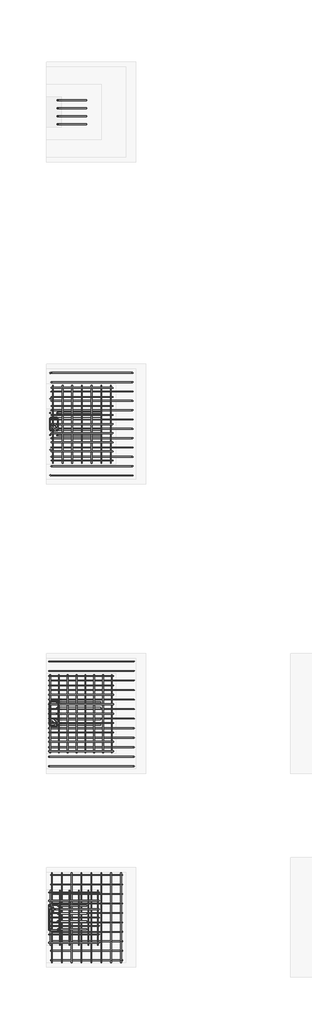
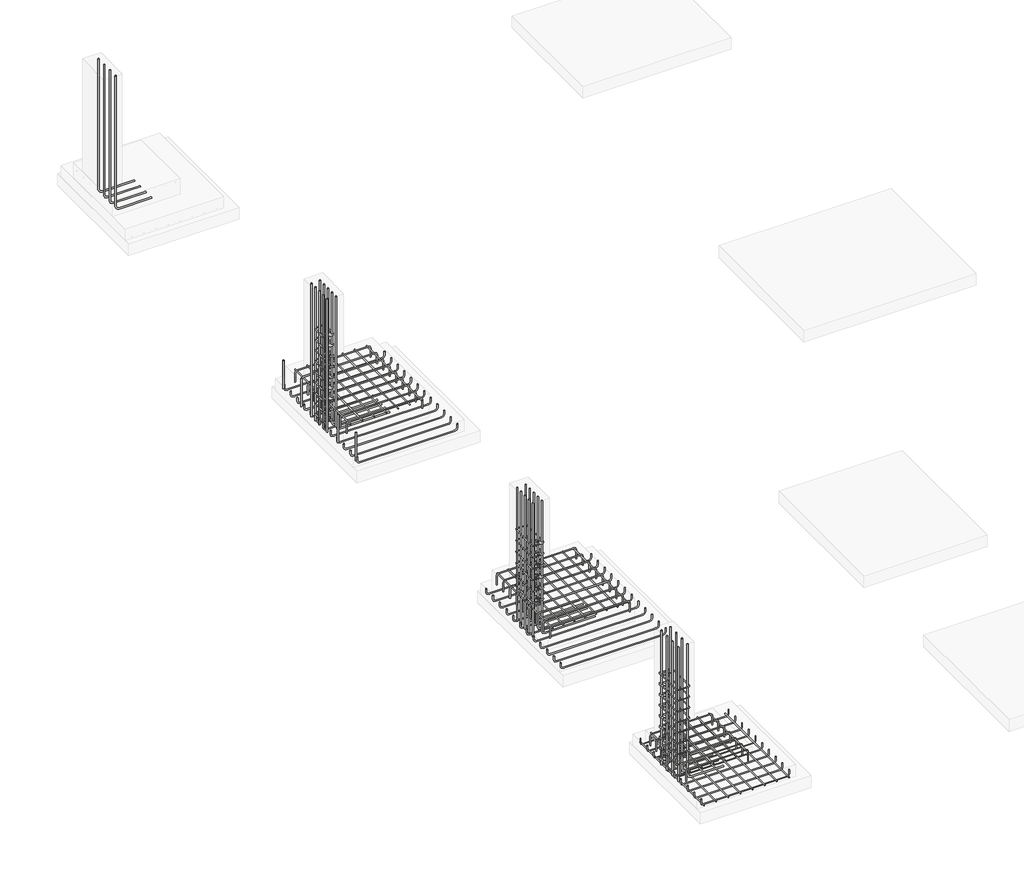
# One storey, part 2 of 6: 21 reinforcing bars.
"""IFC4 building model written with IfcOpenShell, lengths in millimetres."""

from ifc_helpers import new_model, si_unit, point, frame, origin, place, context, project, spatial, polyline, circle_curve, trimmed, segment, composite_curve, source, transform, mapped, element, save
from ifc_brep_helpers import swept_disk

model = new_model("IFC4")

# Units and contexts
model_context = context("Model", 3, world=origin())
ifc_project = project(units=[si_unit("LENGTHUNIT", "METRE", prefix="MILLI")], contexts=[model_context])

# Site, building, storey
site = spatial("IfcSite", under=ifc_project)
building = spatial("IfcBuilding", under=site)
storey = spatial("IfcBuildingStorey", under=building, Elevation=-1828.8)

# Reinforcing bars
placement = place(None, origin())
reinforcing_bar_shape = source(origin(), model_context, "Body", "SolidModel", [
    swept_disk(composite_curve([segment(polyline([(5663595.3113073, -3589696.1284482, -1571.6), (5663595.3113073, -3589696.1284482, -1457.6)]), True, "CONTINUOUS"), segment(trimmed(circle_curve(frame((5663565.3113073, -3589696.1284482, -1457.6), z_axis=(0.0, -1.0, 0.0), x_axis=(30.0, 0.0, 0.0)), 30.0), [point((5663595.3113073, -3589696.1284482, -1457.6))], [point((5663565.3113073, -3589696.1284482, -1427.6))], True, "CARTESIAN"), True, "CONTINUOUS"), segment(polyline([(5663565.3113073, -3589696.1284482, -1427.6), (5662690.0789718, -3589696.1284482, -1427.6)]), True, "CONTINUOUS"), segment(trimmed(circle_curve(frame((5662690.0789718, -3589696.1284482, -1457.6), z_axis=(0.0, -1.0, 0.0), x_axis=(0.0, 0.0, 30.0)), 30.0), [point((5662690.0789718, -3589696.1284482, -1427.6))], [point((5662660.0789718, -3589696.1284482, -1457.6))], True, "CARTESIAN"), True, "CONTINUOUS"), segment(polyline([(5662660.0789718, -3589696.1284482, -1457.6), (5662660.0789718, -3589696.1284482, -1571.6)]), True, "CONTINUOUS")], self_intersect=False), 6.0),
])
element("IfcReinforcingBar", 1, at=placement, inside=storey, context=model_context, shape_type="MappedRepresentation", body=[
    mapped(reinforcing_bar_shape, transform((0.0, 0.0, 0.0), x_axis=(1.0, 0.0, 0.0), y_axis=(0.0, 1.0, 0.0), z_axis=(0.0, 0.0, 1.0))),
    mapped(reinforcing_bar_shape, transform((0.0, -138.4, 0.0), x_axis=(1.0, 0.0, 0.0), y_axis=(0.0, 1.0, 0.0), z_axis=(0.0, 0.0, 1.0))),
    mapped(reinforcing_bar_shape, transform((0.0, -276.8, 0.0), x_axis=(1.0, 0.0, 0.0), y_axis=(0.0, 1.0, 0.0), z_axis=(0.0, 0.0, 1.0))),
    mapped(reinforcing_bar_shape, transform((0.0, -415.2, 0.0), x_axis=(1.0, 0.0, 0.0), y_axis=(0.0, 1.0, 0.0), z_axis=(0.0, 0.0, 1.0))),
    mapped(reinforcing_bar_shape, transform((0.0, -553.6, 0.0), x_axis=(1.0, 0.0, 0.0), y_axis=(0.0, 1.0, 0.0), z_axis=(0.0, 0.0, 1.0))),
    mapped(reinforcing_bar_shape, transform((0.0, -692.0, 0.0), x_axis=(1.0, 0.0, 0.0), y_axis=(0.0, 1.0, 0.0), z_axis=(0.0, 0.0, 1.0))),
    mapped(reinforcing_bar_shape, transform((0.0, -830.4, 0.0), x_axis=(1.0, 0.0, 0.0), y_axis=(0.0, 1.0, 0.0), z_axis=(0.0, 0.0, 1.0))),
    mapped(reinforcing_bar_shape, transform((0.0, -968.8, 0.0), x_axis=(1.0, 0.0, 0.0), y_axis=(0.0, 1.0, 0.0), z_axis=(0.0, 0.0, 1.0))),
    mapped(reinforcing_bar_shape, transform((0.0, -1107.2, 0.0), x_axis=(1.0, 0.0, 0.0), y_axis=(0.0, 1.0, 0.0), z_axis=(0.0, 0.0, 1.0))),
])
reinforcing_bar_2_shape = source(origin(), model_context, "Body", "SolidModel", [
    swept_disk(composite_curve([segment(polyline([(5663568.7965546, -3589656.6584405, -1439.5588801), (5663568.7965546, -3590844.2228659, -1439.5588801)]), True, "CONTINUOUS")], self_intersect=False), 6.0),
])
element("IfcReinforcingBar", 2, at=placement, inside=storey, context=model_context, shape_type="MappedRepresentation", body=[
    mapped(reinforcing_bar_2_shape, transform((0.0, 0.0, 0.0), x_axis=(1.0, 0.0, 0.0), y_axis=(0.0, 1.0, 0.0), z_axis=(0.0, 0.0, 1.0))),
    mapped(reinforcing_bar_2_shape, transform((-147.5988176, 0.0, 0.0), x_axis=(1.0, 0.0, 0.0), y_axis=(0.0, 1.0, 0.0), z_axis=(0.0, 0.0, 1.0))),
    mapped(reinforcing_bar_2_shape, transform((-295.1976351, 0.0, 0.0), x_axis=(1.0, 0.0, 0.0), y_axis=(0.0, 1.0, 0.0), z_axis=(0.0, 0.0, 1.0))),
    mapped(reinforcing_bar_2_shape, transform((-442.7964527, 0.0, 0.0), x_axis=(1.0, 0.0, 0.0), y_axis=(0.0, 1.0, 0.0), z_axis=(0.0, 0.0, 1.0))),
    mapped(reinforcing_bar_2_shape, transform((-590.3952702, 0.0, 0.0), x_axis=(1.0, 0.0, 0.0), y_axis=(0.0, 1.0, 0.0), z_axis=(0.0, 0.0, 1.0))),
    mapped(reinforcing_bar_2_shape, transform((-737.9940878, 0.0, 0.0), x_axis=(1.0, 0.0, 0.0), y_axis=(0.0, 1.0, 0.0), z_axis=(0.0, 0.0, 1.0))),
    mapped(reinforcing_bar_2_shape, transform((-885.5929054, 0.0, 0.0), x_axis=(1.0, 0.0, 0.0), y_axis=(0.0, 1.0, 0.0), z_axis=(0.0, 0.0, 1.0))),
])
reinforcing_bar_3_shape = source(origin(), model_context, "Body", "SolidModel", [
    swept_disk(composite_curve([segment(polyline([(5662620.5113073, -3595238.8523052, -1551.6), (5662620.5113073, -3595238.8523052, -1437.6)]), True, "CONTINUOUS"), segment(trimmed(circle_curve(frame((5662650.5113073, -3595238.8523052, -1437.6), z_axis=(0.0, 1.0, 0.0), x_axis=(-30.0, 0.0, 0.0)), 30.0), [point((5662620.5113073, -3595238.8523052, -1437.6))], [point((5662650.5113073, -3595238.8523052, -1407.6))], True, "CARTESIAN"), True, "CONTINUOUS"), segment(polyline([(5662650.5113073, -3595238.8523052, -1407.6), (5663575.9557483, -3595238.8523052, -1407.6)]), True, "CONTINUOUS"), segment(trimmed(circle_curve(frame((5663575.9557483, -3595238.8523052, -1437.6), z_axis=(0.0, 1.0, 0.0), x_axis=(0.0, 0.0, 30.0)), 30.0), [point((5663575.9557483, -3595238.8523052, -1407.6))], [point((5663605.9557483, -3595238.8523052, -1437.6))], True, "CARTESIAN"), True, "CONTINUOUS"), segment(polyline([(5663605.9557483, -3595238.8523052, -1437.6), (5663605.9557483, -3595238.8523052, -1551.6)]), True, "CONTINUOUS")], self_intersect=False), 6.0),
])
element("IfcReinforcingBar", 3, at=placement, inside=storey, context=model_context, shape_type="MappedRepresentation", body=[
    mapped(reinforcing_bar_3_shape, transform((0.0, 0.0, 0.0), x_axis=(1.0, 0.0, 0.0), y_axis=(0.0, 1.0, 0.0), z_axis=(0.0, 0.0, 1.0))),
    mapped(reinforcing_bar_3_shape, transform((0.0, 143.4, 0.0), x_axis=(1.0, 0.0, 0.0), y_axis=(0.0, 1.0, 0.0), z_axis=(0.0, 0.0, 1.0))),
    mapped(reinforcing_bar_3_shape, transform((0.0, 286.8, 0.0), x_axis=(1.0, 0.0, 0.0), y_axis=(0.0, 1.0, 0.0), z_axis=(0.0, 0.0, 1.0))),
    mapped(reinforcing_bar_3_shape, transform((0.0, 430.2, 0.0), x_axis=(1.0, 0.0, 0.0), y_axis=(0.0, 1.0, 0.0), z_axis=(0.0, 0.0, 1.0))),
    mapped(reinforcing_bar_3_shape, transform((0.0, 573.6, 0.0), x_axis=(1.0, 0.0, 0.0), y_axis=(0.0, 1.0, 0.0), z_axis=(0.0, 0.0, 1.0))),
    mapped(reinforcing_bar_3_shape, transform((0.0, 717.0, 0.0), x_axis=(1.0, 0.0, 0.0), y_axis=(0.0, 1.0, 0.0), z_axis=(0.0, 0.0, 1.0))),
    mapped(reinforcing_bar_3_shape, transform((0.0, 860.4, 0.0), x_axis=(1.0, 0.0, 0.0), y_axis=(0.0, 1.0, 0.0), z_axis=(0.0, 0.0, 1.0))),
    mapped(reinforcing_bar_3_shape, transform((0.0, 1003.8, 0.0), x_axis=(1.0, 0.0, 0.0), y_axis=(0.0, 1.0, 0.0), z_axis=(0.0, 0.0, 1.0))),
    mapped(reinforcing_bar_3_shape, transform((0.0, 1147.2, 0.0), x_axis=(1.0, 0.0, 0.0), y_axis=(0.0, 1.0, 0.0), z_axis=(0.0, 0.0, 1.0))),
])
reinforcing_bar_4_shape = source(origin(), model_context, "Body", "SolidModel", [
    swept_disk(composite_curve([segment(polyline([(5662641.1545158, -3595258.3223129, -1419.7151301), (5662641.1545158, -3594070.7578875, -1419.7151301)]), True, "CONTINUOUS")], self_intersect=False), 6.0),
])
element("IfcReinforcingBar", 4, at=placement, inside=storey, context=model_context, shape_type="MappedRepresentation", body=[
    mapped(reinforcing_bar_4_shape, transform((0.0, 0.0, 0.0), x_axis=(1.0, 0.0, 0.0), y_axis=(0.0, 1.0, 0.0), z_axis=(0.0, 0.0, 1.0))),
    mapped(reinforcing_bar_4_shape, transform((134.3834574, 0.0, 0.0), x_axis=(1.0, 0.0, 0.0), y_axis=(0.0, 1.0, 0.0), z_axis=(0.0, 0.0, 1.0))),
    mapped(reinforcing_bar_4_shape, transform((268.7669147, 0.0, 0.0), x_axis=(1.0, 0.0, 0.0), y_axis=(0.0, 1.0, 0.0), z_axis=(0.0, 0.0, 1.0))),
    mapped(reinforcing_bar_4_shape, transform((403.1503721, 0.0, 0.0), x_axis=(1.0, 0.0, 0.0), y_axis=(0.0, 1.0, 0.0), z_axis=(0.0, 0.0, 1.0))),
    mapped(reinforcing_bar_4_shape, transform((537.5338294, 0.0, 0.0), x_axis=(1.0, 0.0, 0.0), y_axis=(0.0, 1.0, 0.0), z_axis=(0.0, 0.0, 1.0))),
    mapped(reinforcing_bar_4_shape, transform((671.9172868, 0.0, 0.0), x_axis=(1.0, 0.0, 0.0), y_axis=(0.0, 1.0, 0.0), z_axis=(0.0, 0.0, 1.0))),
    mapped(reinforcing_bar_4_shape, transform((806.3007441, 0.0, 0.0), x_axis=(1.0, 0.0, 0.0), y_axis=(0.0, 1.0, 0.0), z_axis=(0.0, 0.0, 1.0))),
    mapped(reinforcing_bar_4_shape, transform((940.6842015, 0.0, 0.0), x_axis=(1.0, 0.0, 0.0), y_axis=(0.0, 1.0, 0.0), z_axis=(0.0, 0.0, 1.0))),
])
reinforcing_bar_5_shape = source(origin(), model_context, "Body", "SolidModel", [
    swept_disk(composite_curve([segment(polyline([(5662620.5113073, -3593868.6554739, -1738.0317047), (5662620.5113073, -3593868.6554739, -1787.0317047)]), True, "CONTINUOUS"), segment(trimmed(circle_curve(frame((5662650.5113073, -3593868.6554739, -1787.0317047), z_axis=(0.0, -1.0, 0.0), x_axis=(-30.0, 0.0, 0.0)), 30.0), [point((5662620.5113073, -3593868.6554739, -1787.0317047))], [point((5662650.5113073, -3593868.6554739, -1817.0317047))], True, "CARTESIAN"), True, "CONTINUOUS"), segment(polyline([(5662650.5113073, -3593868.6554739, -1817.0317047), (5663890.1113073, -3593868.6554739, -1817.0317047)]), True, "CONTINUOUS"), segment(trimmed(circle_curve(frame((5663890.1113073, -3593868.6554739, -1787.0317047), z_axis=(0.0, -1.0, 0.0), x_axis=(0.0, 0.0, -30.0)), 30.0), [point((5663890.1113073, -3593868.6554739, -1817.0317047))], [point((5663920.1113073, -3593868.6554739, -1787.0317047))], True, "CARTESIAN"), True, "CONTINUOUS"), segment(polyline([(5663920.1113073, -3593868.6554739, -1787.0317047), (5663920.1113073, -3593868.6554739, -1738.0317047)]), True, "CONTINUOUS")], self_intersect=False), 6.0),
])
element("IfcReinforcingBar", 5, at=placement, inside=storey, context=model_context, shape_type="MappedRepresentation", body=[
    mapped(reinforcing_bar_5_shape, transform((0.0, 0.0, 0.0), x_axis=(1.0, 0.0, 0.0), y_axis=(0.0, 1.0, 0.0), z_axis=(0.0, 0.0, 1.0))),
    mapped(reinforcing_bar_5_shape, transform((0.0, -145.3451665, 0.0), x_axis=(1.0, 0.0, 0.0), y_axis=(0.0, 1.0, 0.0), z_axis=(0.0, 0.0, 1.0))),
    mapped(reinforcing_bar_5_shape, transform((0.0, -290.690333, 0.0), x_axis=(1.0, 0.0, 0.0), y_axis=(0.0, 1.0, 0.0), z_axis=(0.0, 0.0, 1.0))),
    mapped(reinforcing_bar_5_shape, transform((0.0, -436.0354994, 0.0), x_axis=(1.0, 0.0, 0.0), y_axis=(0.0, 1.0, 0.0), z_axis=(0.0, 0.0, 1.0))),
    mapped(reinforcing_bar_5_shape, transform((0.0, -581.3806659, 0.0), x_axis=(1.0, 0.0, 0.0), y_axis=(0.0, 1.0, 0.0), z_axis=(0.0, 0.0, 1.0))),
    mapped(reinforcing_bar_5_shape, transform((0.0, -726.7258324, 0.0), x_axis=(1.0, 0.0, 0.0), y_axis=(0.0, 1.0, 0.0), z_axis=(0.0, 0.0, 1.0))),
    mapped(reinforcing_bar_5_shape, transform((0.0, -872.0709989, 0.0), x_axis=(1.0, 0.0, 0.0), y_axis=(0.0, 1.0, 0.0), z_axis=(0.0, 0.0, 1.0))),
    mapped(reinforcing_bar_5_shape, transform((0.0, -1017.4161654, 0.0), x_axis=(1.0, 0.0, 0.0), y_axis=(0.0, 1.0, 0.0), z_axis=(0.0, 0.0, 1.0))),
    mapped(reinforcing_bar_5_shape, transform((0.0, -1162.7613318, 0.0), x_axis=(1.0, 0.0, 0.0), y_axis=(0.0, 1.0, 0.0), z_axis=(0.0, 0.0, 1.0))),
    mapped(reinforcing_bar_5_shape, transform((0.0, -1308.1064983, 0.0), x_axis=(1.0, 0.0, 0.0), y_axis=(0.0, 1.0, 0.0), z_axis=(0.0, 0.0, 1.0))),
    mapped(reinforcing_bar_5_shape, transform((0.0, -1453.4516648, 0.0), x_axis=(1.0, 0.0, 0.0), y_axis=(0.0, 1.0, 0.0), z_axis=(0.0, 0.0, 1.0))),
    mapped(reinforcing_bar_5_shape, transform((0.0, -1598.7968313, 0.0), x_axis=(1.0, 0.0, 0.0), y_axis=(0.0, 1.0, 0.0), z_axis=(0.0, 0.0, 1.0))),
])
reinforcing_bar_6_shape = source(origin(), model_context, "Body", "SolidModel", [
    swept_disk(composite_curve([segment(polyline([(5662651.6237213, -3597125.2875145, -1738.4709043), (5662651.6237213, -3597125.2875145, -1793.4709043)]), True, "CONTINUOUS"), segment(trimmed(circle_curve(frame((5662676.6237213, -3597125.2875145, -1793.4709043), z_axis=(0.0, -1.0, 0.0), x_axis=(-25.0, 0.0, 0.0)), 25.0), [point((5662651.6237213, -3597125.2875145, -1793.4709043))], [point((5662676.6237213, -3597125.2875145, -1818.4709043))], True, "CARTESIAN"), True, "CONTINUOUS"), segment(polyline([(5662676.6237213, -3597125.2875145, -1818.4709043), (5663718.1378894, -3597125.2875145, -1818.4709043)]), True, "CONTINUOUS"), segment(trimmed(circle_curve(frame((5663718.1378894, -3597125.2875145, -1793.4709043), z_axis=(0.0, -1.0, 0.0), x_axis=(0.0, 0.0, -25.0)), 25.0), [point((5663718.1378894, -3597125.2875145, -1818.4709043))], [point((5663743.1378894, -3597125.2875145, -1793.4709043))], True, "CARTESIAN"), True, "CONTINUOUS"), segment(polyline([(5663743.1378894, -3597125.2875145, -1793.4709043), (5663743.1378894, -3597125.2875145, -1738.4709043)]), True, "CONTINUOUS")], self_intersect=False), 5.0),
])
element("IfcReinforcingBar", 6, at=placement, inside=storey, context=model_context, shape_type="MappedRepresentation", body=[
    mapped(reinforcing_bar_6_shape, transform((0.0, 0.0, 0.0), x_axis=(1.0, 0.0, 0.0), y_axis=(0.0, 1.0, 0.0), z_axis=(0.0, 0.0, 1.0))),
    mapped(reinforcing_bar_6_shape, transform((0.0, -144.6222222, 0.0), x_axis=(1.0, 0.0, 0.0), y_axis=(0.0, 1.0, 0.0), z_axis=(0.0, 0.0, 1.0))),
    mapped(reinforcing_bar_6_shape, transform((0.0, -289.2444444, 0.0), x_axis=(1.0, 0.0, 0.0), y_axis=(0.0, 1.0, 0.0), z_axis=(0.0, 0.0, 1.0))),
    mapped(reinforcing_bar_6_shape, transform((0.0, -433.8666667, 0.0), x_axis=(1.0, 0.0, 0.0), y_axis=(0.0, 1.0, 0.0), z_axis=(0.0, 0.0, 1.0))),
    mapped(reinforcing_bar_6_shape, transform((0.0, -578.4888889, 0.0), x_axis=(1.0, 0.0, 0.0), y_axis=(0.0, 1.0, 0.0), z_axis=(0.0, 0.0, 1.0))),
    mapped(reinforcing_bar_6_shape, transform((0.0, -723.1111111, 0.0), x_axis=(1.0, 0.0, 0.0), y_axis=(0.0, 1.0, 0.0), z_axis=(0.0, 0.0, 1.0))),
    mapped(reinforcing_bar_6_shape, transform((0.0, -867.7333333, 0.0), x_axis=(1.0, 0.0, 0.0), y_axis=(0.0, 1.0, 0.0), z_axis=(0.0, 0.0, 1.0))),
    mapped(reinforcing_bar_6_shape, transform((0.0, -1012.3555556, 0.0), x_axis=(1.0, 0.0, 0.0), y_axis=(0.0, 1.0, 0.0), z_axis=(0.0, 0.0, 1.0))),
    mapped(reinforcing_bar_6_shape, transform((0.0, -1156.9777778, 0.0), x_axis=(1.0, 0.0, 0.0), y_axis=(0.0, 1.0, 0.0), z_axis=(0.0, 0.0, 1.0))),
    mapped(reinforcing_bar_6_shape, transform((0.0, -1301.6, 0.0), x_axis=(1.0, 0.0, 0.0), y_axis=(0.0, 1.0, 0.0), z_axis=(0.0, 0.0, 1.0))),
])
reinforcing_bar_7_shape = source(origin(), model_context, "Body", "SolidModel", [
    swept_disk(composite_curve([segment(polyline([(5662668.193273, -3597090.2875145, -1807.7638193), (5662668.193273, -3598461.8875145, -1807.7638193)]), True, "CONTINUOUS")], self_intersect=False), 5.0),
])
element("IfcReinforcingBar", 7, at=placement, inside=storey, context=model_context, shape_type="MappedRepresentation", body=[
    mapped(reinforcing_bar_7_shape, transform((0.0, 0.0, 0.0), x_axis=(1.0, 0.0, 0.0), y_axis=(0.0, 1.0, 0.0), z_axis=(0.0, 0.0, 1.0))),
    mapped(reinforcing_bar_7_shape, transform((150.6667583, 0.0, 0.0), x_axis=(1.0, 0.0, 0.0), y_axis=(0.0, 1.0, 0.0), z_axis=(0.0, 0.0, 1.0))),
    mapped(reinforcing_bar_7_shape, transform((301.3335165, 0.0, 0.0), x_axis=(1.0, 0.0, 0.0), y_axis=(0.0, 1.0, 0.0), z_axis=(0.0, 0.0, 1.0))),
    mapped(reinforcing_bar_7_shape, transform((452.0002748, 0.0, 0.0), x_axis=(1.0, 0.0, 0.0), y_axis=(0.0, 1.0, 0.0), z_axis=(0.0, 0.0, 1.0))),
    mapped(reinforcing_bar_7_shape, transform((602.6670331, 0.0, 0.0), x_axis=(1.0, 0.0, 0.0), y_axis=(0.0, 1.0, 0.0), z_axis=(0.0, 0.0, 1.0))),
    mapped(reinforcing_bar_7_shape, transform((753.3337913, 0.0, 0.0), x_axis=(1.0, 0.0, 0.0), y_axis=(0.0, 1.0, 0.0), z_axis=(0.0, 0.0, 1.0))),
    mapped(reinforcing_bar_7_shape, transform((904.0005496, 0.0, 0.0), x_axis=(1.0, 0.0, 0.0), y_axis=(0.0, 1.0, 0.0), z_axis=(0.0, 0.0, 1.0))),
    mapped(reinforcing_bar_7_shape, transform((1054.6673079, 0.0, 0.0), x_axis=(1.0, 0.0, 0.0), y_axis=(0.0, 1.0, 0.0), z_axis=(0.0, 0.0, 1.0))),
])
reinforcing_bar_8_shape = source(origin(), model_context, "Body", "SolidModel", [
    swept_disk(composite_curve([segment(polyline([(5662657.3977763, -3589467.5284482, -1743.8), (5662657.3977763, -3589467.5284482, -1792.8)]), True, "CONTINUOUS"), segment(trimmed(circle_curve(frame((5662687.3977763, -3589467.5284482, -1792.8), z_axis=(0.0, -1.0, 0.0), x_axis=(-30.0, 0.0, 0.0)), 30.0), [point((5662657.3977763, -3589467.5284482, -1792.8))], [point((5662687.3977763, -3589467.5284482, -1822.8))], True, "CARTESIAN"), True, "CONTINUOUS"), segment(polyline([(5662687.3977763, -3589467.5284482, -1822.8), (5663870.1113073, -3589467.5284482, -1822.8)]), True, "CONTINUOUS"), segment(trimmed(circle_curve(frame((5663870.1113073, -3589467.5284482, -1792.8), z_axis=(0.0, -1.0, 0.0), x_axis=(0.0, 0.0, -30.0)), 30.0), [point((5663870.1113073, -3589467.5284482, -1822.8))], [point((5663900.1113073, -3589467.5284482, -1792.8))], True, "CARTESIAN"), True, "CONTINUOUS"), segment(polyline([(5663900.1113073, -3589467.5284482, -1792.8), (5663900.1113073, -3589467.5284482, -1743.8)]), True, "CONTINUOUS")], self_intersect=False), 6.0),
])
element("IfcReinforcingBar", 8, at=placement, inside=storey, context=model_context, shape_type="MappedRepresentation", body=[
    mapped(reinforcing_bar_8_shape, transform((0.0, 0.0, 0.0), x_axis=(1.0, 0.0, 0.0), y_axis=(0.0, 1.0, 0.0), z_axis=(0.0, 0.0, 1.0))),
    mapped(reinforcing_bar_8_shape, transform((0.0, -142.2181818, 0.0), x_axis=(1.0, 0.0, 0.0), y_axis=(0.0, 1.0, 0.0), z_axis=(0.0, 0.0, 1.0))),
    mapped(reinforcing_bar_8_shape, transform((0.0, -284.4363636, 0.0), x_axis=(1.0, 0.0, 0.0), y_axis=(0.0, 1.0, 0.0), z_axis=(0.0, 0.0, 1.0))),
    mapped(reinforcing_bar_8_shape, transform((0.0, -426.6545455, 0.0), x_axis=(1.0, 0.0, 0.0), y_axis=(0.0, 1.0, 0.0), z_axis=(0.0, 0.0, 1.0))),
    mapped(reinforcing_bar_8_shape, transform((0.0, -568.8727273, 0.0), x_axis=(1.0, 0.0, 0.0), y_axis=(0.0, 1.0, 0.0), z_axis=(0.0, 0.0, 1.0))),
    mapped(reinforcing_bar_8_shape, transform((0.0, -711.0909091, 0.0), x_axis=(1.0, 0.0, 0.0), y_axis=(0.0, 1.0, 0.0), z_axis=(0.0, 0.0, 1.0))),
    mapped(reinforcing_bar_8_shape, transform((0.0, -853.3090909, 0.0), x_axis=(1.0, 0.0, 0.0), y_axis=(0.0, 1.0, 0.0), z_axis=(0.0, 0.0, 1.0))),
    mapped(reinforcing_bar_8_shape, transform((0.0, -995.5272727, 0.0), x_axis=(1.0, 0.0, 0.0), y_axis=(0.0, 1.0, 0.0), z_axis=(0.0, 0.0, 1.0))),
    mapped(reinforcing_bar_8_shape, transform((0.0, -1137.7454545, 0.0), x_axis=(1.0, 0.0, 0.0), y_axis=(0.0, 1.0, 0.0), z_axis=(0.0, 0.0, 1.0))),
    mapped(reinforcing_bar_8_shape, transform((0.0, -1279.9636364, 0.0), x_axis=(1.0, 0.0, 0.0), y_axis=(0.0, 1.0, 0.0), z_axis=(0.0, 0.0, 1.0))),
    mapped(reinforcing_bar_8_shape, transform((0.0, -1422.1818182, 0.0), x_axis=(1.0, 0.0, 0.0), y_axis=(0.0, 1.0, 0.0), z_axis=(0.0, 0.0, 1.0))),
    mapped(reinforcing_bar_8_shape, transform((0.0, -1564.4, 0.0), x_axis=(1.0, 0.0, 0.0), y_axis=(0.0, 1.0, 0.0), z_axis=(0.0, 0.0, 1.0))),
])
reinforcing_bar_9_shape = source(origin(), model_context, "Body", "SolidModel", [
    swept_disk(composite_curve([segment(polyline([(5662749.6650571, -3590077.0682909, -40.0), (5662749.6650571, -3590077.0682909, -1746.25)]), True, "CONTINUOUS"), segment(trimmed(circle_curve(frame((5662789.6650571, -3590077.0682909, -1746.25), z_axis=(0.0, -1.0, 0.0), x_axis=(-40.0, 0.0, 0.0)), 40.0), [point((5662749.6650571, -3590077.0682909, -1746.25))], [point((5662789.6650571, -3590077.0682909, -1786.25))], True, "CARTESIAN"), True, "CONTINUOUS"), segment(polyline([(5662789.6650571, -3590077.0682909, -1786.25), (5663410.0650571, -3590077.0682909, -1786.25)]), True, "CONTINUOUS")], self_intersect=False), 8.0),
])
element("IfcReinforcingBar", 9, at=placement, inside=storey, context=model_context, shape_type="MappedRepresentation", body=[
    mapped(reinforcing_bar_9_shape, transform((0.0, 0.0, 0.0), x_axis=(1.0, 0.0, 0.0), y_axis=(0.0, 1.0, 0.0), z_axis=(0.0, 0.0, 1.0))),
    mapped(reinforcing_bar_9_shape, transform((0.0, -86.3, 0.0), x_axis=(1.0, 0.0, 0.0), y_axis=(0.0, 1.0, 0.0), z_axis=(0.0, 0.0, 1.0))),
    mapped(reinforcing_bar_9_shape, transform((0.0, -172.6, 0.0), x_axis=(1.0, 0.0, 0.0), y_axis=(0.0, 1.0, 0.0), z_axis=(0.0, 0.0, 1.0))),
    mapped(reinforcing_bar_9_shape, transform((0.0, -258.9, 0.0), x_axis=(1.0, 0.0, 0.0), y_axis=(0.0, 1.0, 0.0), z_axis=(0.0, 0.0, 1.0))),
    mapped(reinforcing_bar_9_shape, transform((0.0, -345.2, 0.0), x_axis=(1.0, 0.0, 0.0), y_axis=(0.0, 1.0, 0.0), z_axis=(0.0, 0.0, 1.0))),
])
reinforcing_bar_10_shape = source(origin(), model_context, "Body", "SolidModel", [
    swept_disk(composite_curve([segment(polyline([(5662642.9082028, -3590079.4114367, -40.0), (5662642.9082028, -3590079.4114367, -1787.5415145)]), True, "CONTINUOUS")], self_intersect=False), 8.0),
])
element("IfcReinforcingBar", 10, at=placement, inside=storey, context=model_context, shape_type="MappedRepresentation", body=[
    mapped(reinforcing_bar_10_shape, transform((0.0, 0.0, 0.0), x_axis=(1.0, 0.0, 0.0), y_axis=(0.0, 1.0, 0.0), z_axis=(0.0, 0.0, 1.0))),
    mapped(reinforcing_bar_10_shape, transform((0.0, -83.7142136, 0.0), x_axis=(1.0, 0.0, 0.0), y_axis=(0.0, 1.0, 0.0), z_axis=(0.0, 0.0, 1.0))),
    mapped(reinforcing_bar_10_shape, transform((0.0, -167.4284271, 0.0), x_axis=(1.0, 0.0, 0.0), y_axis=(0.0, 1.0, 0.0), z_axis=(0.0, 0.0, 1.0))),
    mapped(reinforcing_bar_10_shape, transform((0.0, -251.1426407, 0.0), x_axis=(1.0, 0.0, 0.0), y_axis=(0.0, 1.0, 0.0), z_axis=(0.0, 0.0, 1.0))),
    mapped(reinforcing_bar_10_shape, transform((0.0, -334.8568542, 0.0), x_axis=(1.0, 0.0, 0.0), y_axis=(0.0, 1.0, 0.0), z_axis=(0.0, 0.0, 1.0))),
])
reinforcing_bar_11_shape = source(origin(), model_context, "Body", "SolidModel", [
    swept_disk(composite_curve([segment(polyline([(5662644.5742178, -3589469.5284482, -1787.9128402), (5662644.5742178, -3589469.5284482, -1421.6)]), True, "CONTINUOUS")], self_intersect=False), 8.0),
])
element("IfcReinforcingBar", 11, at=placement, inside=storey, context=model_context, shape_type="MappedRepresentation", body=[
    mapped(reinforcing_bar_11_shape, transform((0.0, 0.0, 0.0), x_axis=(1.0, 0.0, 0.0), y_axis=(0.0, 1.0, 0.0), z_axis=(0.0, 0.0, 1.0))),
    mapped(reinforcing_bar_11_shape, transform((0.0, -390.1, 0.0), x_axis=(1.0, 0.0, 0.0), y_axis=(0.0, 1.0, 0.0), z_axis=(0.0, 0.0, 1.0))),
    mapped(reinforcing_bar_11_shape, transform((0.0, -780.2, 0.0), x_axis=(1.0, 0.0, 0.0), y_axis=(0.0, 1.0, 0.0), z_axis=(0.0, 0.0, 1.0))),
    mapped(reinforcing_bar_11_shape, transform((0.0, -1170.3, 0.0), x_axis=(1.0, 0.0, 0.0), y_axis=(0.0, 1.0, 0.0), z_axis=(0.0, 0.0, 1.0))),
    mapped(reinforcing_bar_11_shape, transform((0.0, -1560.4, 0.0), x_axis=(1.0, 0.0, 0.0), y_axis=(0.0, 1.0, 0.0), z_axis=(0.0, 0.0, 1.0))),
])
reinforcing_bar_12_shape = source(origin(), model_context, "Body", "SolidModel", [
    swept_disk(composite_curve([segment(polyline([(5662662.6433659, -3590279.9314221, -1695.1328603), (5662726.990083, -3590344.2781392, -1695.1328603)]), True, "CONTINUOUS"), segment(trimmed(circle_curve(frame((5662741.1322186, -3590330.1360036, -1695.1328603), z_axis=(0.0, 0.0, 1.0), x_axis=(-14.142135600559413, -14.142135600093752, 0.0)), 20.0), [point((5662726.990083, -3590344.2781392, -1695.1328603))], [point((5662761.1322186, -3590330.1360036, -1695.1328603))], True, "CARTESIAN"), True, "CONTINUOUS"), segment(polyline([(5662761.1322186, -3590330.1360036, -1695.1328603), (5662761.1322186, -3590169.3127555, -1695.1328603)]), True, "CONTINUOUS"), segment(trimmed(circle_curve(frame((5662741.1322186, -3590169.3127555, -1695.1328603), z_axis=(0.0, 0.0, 1.0), x_axis=(20.0, 0.0, 0.0)), 20.0), [point((5662761.1322186, -3590169.3127555, -1695.1328603))], [point((5662741.1322186, -3590149.3127555, -1695.1328603))], True, "CARTESIAN"), True, "CONTINUOUS"), segment(polyline([(5662741.1322186, -3590149.3127555, -1695.1328603), (5662657.0905272, -3590149.3127555, -1695.1328603)]), True, "CONTINUOUS"), segment(trimmed(circle_curve(frame((5662657.0905272, -3590169.2969053, -1695.9289494), z_axis=(0.0, -0.03980445484139933, 0.9992074886502698), x_axis=(0.0, 19.98414980014786, 0.7960891000000174)), 20.0), [point((5662657.0905272, -3590149.3127555, -1695.1328603))], [point((5662637.0905272, -3590169.2969053, -1695.9289494))], True, "CARTESIAN"), True, "CONTINUOUS"), segment(polyline([(5662637.0905272, -3590169.2969053, -1695.9289494), (5662637.0905272, -3590330.1518538, -1702.3367712)]), True, "CONTINUOUS"), segment(trimmed(circle_curve(frame((5662657.0905272, -3590330.1518538, -1702.3367712), z_axis=(0.0, -0.03980445484139933, 0.9992074886502698), x_axis=(-20.0, 0.0, 0.0)), 20.0), [point((5662637.0905272, -3590330.1518538, -1702.3367712))], [point((5662657.0905272, -3590350.1360036, -1703.1328603))], True, "CARTESIAN"), True, "CONTINUOUS"), segment(polyline([(5662657.0905272, -3590350.1360036, -1703.1328603), (5662741.1322186, -3590350.1360036, -1703.1328603)]), True, "CONTINUOUS"), segment(trimmed(circle_curve(frame((5662741.1322186, -3590330.1360036, -1703.1328603), z_axis=(0.0, 0.0, 1.0), x_axis=(0.0, -20.0, 0.0)), 20.0), [point((5662741.1322186, -3590350.1360036, -1703.1328603))], [point((5662755.2743542, -3590315.993868, -1703.1328603))], True, "CARTESIAN"), True, "CONTINUOUS"), segment(polyline([(5662755.2743542, -3590315.993868, -1703.1328603), (5662690.9276371, -3590251.6471509, -1703.1328603)]), True, "CONTINUOUS")], self_intersect=False), 4.0),
])
element("IfcReinforcingBar", 12, at=placement, inside=storey, context=model_context, shape_type="MappedRepresentation", body=[
    mapped(reinforcing_bar_12_shape, transform((0.0, 0.0, 0.0), x_axis=(1.0, 0.0, 0.0), y_axis=(0.0, 1.0, 0.0), z_axis=(0.0, 0.0, 1.0))),
    mapped(reinforcing_bar_12_shape, transform((0.0, 0.0, 138.8666075), x_axis=(1.0, 0.0, 0.0), y_axis=(0.0, 1.0, 0.0), z_axis=(0.0, 0.0, 1.0))),
    mapped(reinforcing_bar_12_shape, transform((0.0, 0.0, 277.7332151), x_axis=(1.0, 0.0, 0.0), y_axis=(0.0, 1.0, 0.0), z_axis=(0.0, 0.0, 1.0))),
    mapped(reinforcing_bar_12_shape, transform((0.0, 0.0, 416.5998226), x_axis=(1.0, 0.0, 0.0), y_axis=(0.0, 1.0, 0.0), z_axis=(0.0, 0.0, 1.0))),
    mapped(reinforcing_bar_12_shape, transform((0.0, 0.0, 555.4664302), x_axis=(1.0, 0.0, 0.0), y_axis=(0.0, 1.0, 0.0), z_axis=(0.0, 0.0, 1.0))),
    mapped(reinforcing_bar_12_shape, transform((0.0, 0.0, 694.3330377), x_axis=(1.0, 0.0, 0.0), y_axis=(0.0, 1.0, 0.0), z_axis=(0.0, 0.0, 1.0))),
    mapped(reinforcing_bar_12_shape, transform((0.0, 0.0, 833.1996452), x_axis=(1.0, 0.0, 0.0), y_axis=(0.0, 1.0, 0.0), z_axis=(0.0, 0.0, 1.0))),
    mapped(reinforcing_bar_12_shape, transform((0.0, 0.0, 972.0662528), x_axis=(1.0, 0.0, 0.0), y_axis=(0.0, 1.0, 0.0), z_axis=(0.0, 0.0, 1.0))),
    mapped(reinforcing_bar_12_shape, transform((0.0, 0.0, 1110.9328603), x_axis=(1.0, 0.0, 0.0), y_axis=(0.0, 1.0, 0.0), z_axis=(0.0, 0.0, 1.0))),
])
reinforcing_bar_13_shape = source(origin(), model_context, "Body", "SolidModel", [
    swept_disk(composite_curve([segment(polyline([(5662749.6650571, -3594492.6523052, -40.0), (5662749.6650571, -3594492.6523052, -1746.25)]), True, "CONTINUOUS"), segment(trimmed(circle_curve(frame((5662789.6650571, -3594492.6523052, -1746.25), z_axis=(0.0, -1.0, 0.0), x_axis=(-40.0, 0.0, 0.0)), 40.0), [point((5662749.6650571, -3594492.6523052, -1746.25))], [point((5662789.6650571, -3594492.6523052, -1786.25))], True, "CARTESIAN"), True, "CONTINUOUS"), segment(polyline([(5662789.6650571, -3594492.6523052, -1786.25), (5663410.0650571, -3594492.6523052, -1786.25)]), True, "CONTINUOUS")], self_intersect=False), 8.0),
])
element("IfcReinforcingBar", 13, at=placement, inside=storey, context=model_context, shape_type="MappedRepresentation", body=[
    mapped(reinforcing_bar_13_shape, transform((0.0, 0.0, 0.0), x_axis=(1.0, 0.0, 0.0), y_axis=(0.0, 1.0, 0.0), z_axis=(0.0, 0.0, 1.0))),
    mapped(reinforcing_bar_13_shape, transform((0.0, -86.3, 0.0), x_axis=(1.0, 0.0, 0.0), y_axis=(0.0, 1.0, 0.0), z_axis=(0.0, 0.0, 1.0))),
    mapped(reinforcing_bar_13_shape, transform((0.0, -172.6, 0.0), x_axis=(1.0, 0.0, 0.0), y_axis=(0.0, 1.0, 0.0), z_axis=(0.0, 0.0, 1.0))),
    mapped(reinforcing_bar_13_shape, transform((0.0, -258.9, 0.0), x_axis=(1.0, 0.0, 0.0), y_axis=(0.0, 1.0, 0.0), z_axis=(0.0, 0.0, 1.0))),
    mapped(reinforcing_bar_13_shape, transform((0.0, -345.2, 0.0), x_axis=(1.0, 0.0, 0.0), y_axis=(0.0, 1.0, 0.0), z_axis=(0.0, 0.0, 1.0))),
])
reinforcing_bar_14_shape = source(origin(), model_context, "Body", "SolidModel", [
    swept_disk(composite_curve([segment(polyline([(5662642.9082028, -3594494.9954509, -40.0), (5662642.9082028, -3594494.9954509, -1787.5415145)]), True, "CONTINUOUS")], self_intersect=False), 8.0),
])
element("IfcReinforcingBar", 14, at=placement, inside=storey, context=model_context, shape_type="MappedRepresentation", body=[
    mapped(reinforcing_bar_14_shape, transform((0.0, 0.0, 0.0), x_axis=(1.0, 0.0, 0.0), y_axis=(0.0, 1.0, 0.0), z_axis=(0.0, 0.0, 1.0))),
    mapped(reinforcing_bar_14_shape, transform((0.0, -83.7142136, 0.0), x_axis=(1.0, 0.0, 0.0), y_axis=(0.0, 1.0, 0.0), z_axis=(0.0, 0.0, 1.0))),
    mapped(reinforcing_bar_14_shape, transform((0.0, -167.4284271, 0.0), x_axis=(1.0, 0.0, 0.0), y_axis=(0.0, 1.0, 0.0), z_axis=(0.0, 0.0, 1.0))),
    mapped(reinforcing_bar_14_shape, transform((0.0, -251.1426407, 0.0), x_axis=(1.0, 0.0, 0.0), y_axis=(0.0, 1.0, 0.0), z_axis=(0.0, 0.0, 1.0))),
    mapped(reinforcing_bar_14_shape, transform((0.0, -334.8568542, 0.0), x_axis=(1.0, 0.0, 0.0), y_axis=(0.0, 1.0, 0.0), z_axis=(0.0, 0.0, 1.0))),
])
reinforcing_bar_15_shape = source(origin(), model_context, "Body", "SolidModel", [
    swept_disk(composite_curve([segment(polyline([(5662670.6762044, -3594779.6477237, -1327.6), (5662735.0229215, -3594843.9944408, -1327.6)]), True, "CONTINUOUS"), segment(trimmed(circle_curve(frame((5662749.1650571, -3594829.8523052, -1327.6), z_axis=(0.0, 0.0, 1.0), x_axis=(-14.142135600559413, -14.142135600093752, 0.0)), 20.0), [point((5662735.0229215, -3594843.9944408, -1327.6))], [point((5662769.1650571, -3594829.8523052, -1327.6))], True, "CARTESIAN"), True, "CONTINUOUS"), segment(polyline([(5662769.1650571, -3594829.8523052, -1327.6), (5662769.1650571, -3594500.6523052, -1327.6)]), True, "CONTINUOUS"), segment(trimmed(circle_curve(frame((5662749.1650571, -3594500.6523052, -1327.6), z_axis=(0.0, 0.0, 1.0), x_axis=(20.0, 0.0, 0.0)), 20.0), [point((5662769.1650571, -3594500.6523052, -1327.6))], [point((5662749.1650571, -3594480.6523052, -1327.6))], True, "CARTESIAN"), True, "CONTINUOUS"), segment(polyline([(5662749.1650571, -3594480.6523052, -1327.6), (5662648.5650571, -3594480.6523052, -1327.6)]), True, "CONTINUOUS"), segment(trimmed(circle_curve(frame((5662648.5650571, -3594500.6476116, -1328.0332677), z_axis=(0.0, -0.021663387243443962, 0.9997653212895218), x_axis=(0.0, 19.99530639965087, 0.4332676999999876)), 20.0), [point((5662648.5650571, -3594480.6523052, -1327.6))], [point((5662628.5650571, -3594500.6476116, -1328.0332677))], True, "CARTESIAN"), True, "CONTINUOUS"), segment(polyline([(5662628.5650571, -3594500.6476116, -1328.0332677), (5662628.5650571, -3594829.8569988, -1335.1667323)]), True, "CONTINUOUS"), segment(trimmed(circle_curve(frame((5662648.5650571, -3594829.8569988, -1335.1667323), z_axis=(0.0, -0.021663387243443962, 0.9997653212895218), x_axis=(-20.0, 0.0, 0.0)), 20.0), [point((5662628.5650571, -3594829.8569988, -1335.1667323))], [point((5662648.5650571, -3594849.8523052, -1335.6))], True, "CARTESIAN"), True, "CONTINUOUS"), segment(polyline([(5662648.5650571, -3594849.8523052, -1335.6), (5662749.1650571, -3594849.8523052, -1335.6)]), True, "CONTINUOUS"), segment(trimmed(circle_curve(frame((5662749.1650571, -3594829.8523052, -1335.6), z_axis=(0.0, 0.0, 1.0), x_axis=(0.0, -20.0, 0.0)), 20.0), [point((5662749.1650571, -3594849.8523052, -1335.6))], [point((5662763.3071927, -3594815.7101696, -1335.6))], True, "CARTESIAN"), True, "CONTINUOUS"), segment(polyline([(5662763.3071927, -3594815.7101696, -1335.6), (5662698.9604756, -3594751.3634525, -1335.6)]), True, "CONTINUOUS")], self_intersect=False), 4.0),
])
element("IfcReinforcingBar", 15, at=placement, inside=storey, context=model_context, shape_type="MappedRepresentation", body=[
    mapped(reinforcing_bar_15_shape, transform((0.0, 0.0, 0.0), x_axis=(1.0, 0.0, 0.0), y_axis=(0.0, 1.0, 0.0), z_axis=(0.0, 0.0, 1.0))),
    mapped(reinforcing_bar_15_shape, transform((0.0, 0.0, 148.68), x_axis=(1.0, 0.0, 0.0), y_axis=(0.0, 1.0, 0.0), z_axis=(0.0, 0.0, 1.0))),
    mapped(reinforcing_bar_15_shape, transform((0.0, 0.0, 297.36), x_axis=(1.0, 0.0, 0.0), y_axis=(0.0, 1.0, 0.0), z_axis=(0.0, 0.0, 1.0))),
    mapped(reinforcing_bar_15_shape, transform((0.0, 0.0, 446.04), x_axis=(1.0, 0.0, 0.0), y_axis=(0.0, 1.0, 0.0), z_axis=(0.0, 0.0, 1.0))),
    mapped(reinforcing_bar_15_shape, transform((0.0, 0.0, 594.72), x_axis=(1.0, 0.0, 0.0), y_axis=(0.0, 1.0, 0.0), z_axis=(0.0, 0.0, 1.0))),
    mapped(reinforcing_bar_15_shape, transform((0.0, 0.0, 743.4), x_axis=(1.0, 0.0, 0.0), y_axis=(0.0, 1.0, 0.0), z_axis=(0.0, 0.0, 1.0))),
])
reinforcing_bar_16_shape = source(origin(), model_context, "Body", "SolidModel", [
    swept_disk(composite_curve([segment(polyline([(5662755.9613073, -3597591.8975754, -30.0), (5662755.9613073, -3597591.8975754, -1742.6)]), True, "CONTINUOUS"), segment(trimmed(circle_curve(frame((5662795.9613073, -3597591.8975754, -1742.6), z_axis=(0.0, -1.0, 0.0), x_axis=(-40.0, 0.0, 0.0)), 40.0), [point((5662755.9613073, -3597591.8975754, -1742.6))], [point((5662795.9613073, -3597591.8975754, -1782.6))], True, "CARTESIAN"), True, "CONTINUOUS"), segment(polyline([(5662795.9613073, -3597591.8975754, -1782.6), (5663200.4613073, -3597591.8975754, -1782.6)]), True, "CONTINUOUS")], self_intersect=False), 8.0),
])
element("IfcReinforcingBar", 16, at=placement, inside=storey, context=model_context, shape_type="MappedRepresentation", body=[
    mapped(reinforcing_bar_16_shape, transform((0.0, 0.0, 0.0), x_axis=(1.0, 0.0, 0.0), y_axis=(0.0, 1.0, 0.0), z_axis=(0.0, 0.0, 1.0))),
    mapped(reinforcing_bar_16_shape, transform((0.0, -121.7333333, 0.0), x_axis=(1.0, 0.0, 0.0), y_axis=(0.0, 1.0, 0.0), z_axis=(0.0, 0.0, 1.0))),
    mapped(reinforcing_bar_16_shape, transform((0.0, -243.4666667, 0.0), x_axis=(1.0, 0.0, 0.0), y_axis=(0.0, 1.0, 0.0), z_axis=(0.0, 0.0, 1.0))),
    mapped(reinforcing_bar_16_shape, transform((0.0, -365.2, 0.0), x_axis=(1.0, 0.0, 0.0), y_axis=(0.0, 1.0, 0.0), z_axis=(0.0, 0.0, 1.0))),
])
reinforcing_bar_17_shape = source(origin(), model_context, "Body", "SolidModel", [
    swept_disk(composite_curve([segment(polyline([(5662641.6613073, -3597594.6836876, -30.0), (5662641.6613073, -3597594.6836876, -1788.95)]), True, "CONTINUOUS")], self_intersect=False), 8.0),
])
element("IfcReinforcingBar", 17, at=placement, inside=storey, context=model_context, shape_type="MappedRepresentation", body=[
    mapped(reinforcing_bar_17_shape, transform((0.0, 0.0, 0.0), x_axis=(1.0, 0.0, 0.0), y_axis=(0.0, 1.0, 0.0), z_axis=(0.0, 0.0, 1.0))),
    mapped(reinforcing_bar_17_shape, transform((0.0, -120.1712362, 0.0), x_axis=(1.0, 0.0, 0.0), y_axis=(0.0, 1.0, 0.0), z_axis=(0.0, 0.0, 1.0))),
    mapped(reinforcing_bar_17_shape, transform((0.0, -240.3424723, 0.0), x_axis=(1.0, 0.0, 0.0), y_axis=(0.0, 1.0, 0.0), z_axis=(0.0, 0.0, 1.0))),
    mapped(reinforcing_bar_17_shape, transform((0.0, -360.5137085, 0.0), x_axis=(1.0, 0.0, 0.0), y_axis=(0.0, 1.0, 0.0), z_axis=(0.0, 0.0, 1.0))),
])
reinforcing_bar_18_shape = source(origin(), model_context, "Body", "SolidModel", [
    swept_disk(composite_curve([segment(polyline([(5663387.7113073, -3597391.9875145, -1653.2), (5663387.7113073, -3597391.9875145, -1533.2)]), True, "CONTINUOUS"), segment(trimmed(circle_curve(frame((5663362.7113073, -3597391.9875145, -1533.2), z_axis=(0.0, -1.0, 0.0), x_axis=(25.0, 0.0, 0.0)), 25.0), [point((5663387.7113073, -3597391.9875145, -1533.2))], [point((5663362.7113073, -3597391.9875145, -1508.2))], True, "CARTESIAN"), True, "CONTINUOUS"), segment(polyline([(5663362.7113073, -3597391.9875145, -1508.2), (5662644.5113073, -3597391.9875145, -1508.2)]), True, "CONTINUOUS"), segment(trimmed(circle_curve(frame((5662644.5113073, -3597391.9875145, -1533.2), z_axis=(0.0, -1.0, 0.0), x_axis=(0.0, 0.0, 25.0)), 25.0), [point((5662644.5113073, -3597391.9875145, -1508.2))], [point((5662619.5113073, -3597391.9875145, -1533.2))], True, "CARTESIAN"), True, "CONTINUOUS"), segment(polyline([(5662619.5113073, -3597391.9875145, -1533.2), (5662619.5113073, -3597391.9875145, -1653.2)]), True, "CONTINUOUS")], self_intersect=False), 5.0),
])
element("IfcReinforcingBar", 18, at=placement, inside=storey, context=model_context, shape_type="MappedRepresentation", body=[
    mapped(reinforcing_bar_18_shape, transform((0.0, 0.0, 0.0), x_axis=(1.0, 0.0, 0.0), y_axis=(0.0, 1.0, 0.0), z_axis=(0.0, 0.0, 1.0))),
    mapped(reinforcing_bar_18_shape, transform((0.0, -128.0333333, 0.0), x_axis=(1.0, 0.0, 0.0), y_axis=(0.0, 1.0, 0.0), z_axis=(0.0, 0.0, 1.0))),
    mapped(reinforcing_bar_18_shape, transform((0.0, -256.0666667, 0.0), x_axis=(1.0, 0.0, 0.0), y_axis=(0.0, 1.0, 0.0), z_axis=(0.0, 0.0, 1.0))),
    mapped(reinforcing_bar_18_shape, transform((0.0, -384.1, 0.0), x_axis=(1.0, 0.0, 0.0), y_axis=(0.0, 1.0, 0.0), z_axis=(0.0, 0.0, 1.0))),
    mapped(reinforcing_bar_18_shape, transform((0.0, -512.1333333, 0.0), x_axis=(1.0, 0.0, 0.0), y_axis=(0.0, 1.0, 0.0), z_axis=(0.0, 0.0, 1.0))),
    mapped(reinforcing_bar_18_shape, transform((0.0, -640.1666667, 0.0), x_axis=(1.0, 0.0, 0.0), y_axis=(0.0, 1.0, 0.0), z_axis=(0.0, 0.0, 1.0))),
    mapped(reinforcing_bar_18_shape, transform((0.0, -768.2, 0.0), x_axis=(1.0, 0.0, 0.0), y_axis=(0.0, 1.0, 0.0), z_axis=(0.0, 0.0, 1.0))),
])
reinforcing_bar_19_shape = source(origin(), model_context, "Body", "SolidModel", [
    swept_disk(composite_curve([segment(polyline([(5663367.2515256, -3597356.9875145, -1518.4743523), (5663367.2515256, -3598195.1875145, -1518.4743523)]), True, "CONTINUOUS")], self_intersect=False), 5.0),
])
element("IfcReinforcingBar", 19, at=placement, inside=storey, context=model_context, shape_type="MappedRepresentation", body=[
    mapped(reinforcing_bar_19_shape, transform((0.0, 0.0, 0.0), x_axis=(1.0, 0.0, 0.0), y_axis=(0.0, 1.0, 0.0), z_axis=(0.0, 0.0, 1.0))),
    mapped(reinforcing_bar_19_shape, transform((-143.7654959, 0.0, 0.0), x_axis=(1.0, 0.0, 0.0), y_axis=(0.0, 1.0, 0.0), z_axis=(0.0, 0.0, 1.0))),
    mapped(reinforcing_bar_19_shape, transform((-287.5309918, 0.0, 0.0), x_axis=(1.0, 0.0, 0.0), y_axis=(0.0, 1.0, 0.0), z_axis=(0.0, 0.0, 1.0))),
    mapped(reinforcing_bar_19_shape, transform((-431.2964877, 0.0, 0.0), x_axis=(1.0, 0.0, 0.0), y_axis=(0.0, 1.0, 0.0), z_axis=(0.0, 0.0, 1.0))),
    mapped(reinforcing_bar_19_shape, transform((-575.0619837, 0.0, 0.0), x_axis=(1.0, 0.0, 0.0), y_axis=(0.0, 1.0, 0.0), z_axis=(0.0, 0.0, 1.0))),
    mapped(reinforcing_bar_19_shape, transform((-718.8274796, 0.0, 0.0), x_axis=(1.0, 0.0, 0.0), y_axis=(0.0, 1.0, 0.0), z_axis=(0.0, 0.0, 1.0))),
])
reinforcing_bar_20_shape = source(origin(), model_context, "Body", "SolidModel", [
    swept_disk(composite_curve([segment(polyline([(5662717.00016, -3597650.1021568, -1701.76112), (5662652.6534429, -3597585.7554398, -1701.76112)]), True, "CONTINUOUS"), segment(trimmed(circle_curve(frame((5662638.5113073, -3597599.8975754, -1701.76112), z_axis=(0.0, 0.0, 1.0), x_axis=(14.14213559962809, 14.14213559962809, 0.0)), 20.0), [point((5662652.6534429, -3597585.7554398, -1701.76112))], [point((5662618.5113073, -3597599.8975754, -1701.76112))], True, "CARTESIAN"), True, "CONTINUOUS"), segment(polyline([(5662618.5113073, -3597599.8975754, -1701.76112), (5662618.5113073, -3597949.0975754, -1701.76112)]), True, "CONTINUOUS"), segment(trimmed(circle_curve(frame((5662638.5113073, -3597949.0975754, -1701.76112), z_axis=(0.0, 0.0, 1.0), x_axis=(-20.0, 0.0, 0.0)), 20.0), [point((5662618.5113073, -3597949.0975754, -1701.76112))], [point((5662638.5113073, -3597969.0975754, -1701.76112))], True, "CARTESIAN"), True, "CONTINUOUS"), segment(polyline([(5662638.5113073, -3597969.0975754, -1701.76112), (5662759.1113073, -3597969.0975754, -1701.76112)]), True, "CONTINUOUS"), segment(trimmed(circle_curve(frame((5662759.1113073, -3597949.1017991, -1702.1721329), z_axis=(0.0, 0.020550643642841034, 0.9997888132230052), x_axis=(0.0, -19.995776299852878, 0.41101290000005974)), 20.0), [point((5662759.1113073, -3597969.0975754, -1701.76112))], [point((5662779.1113073, -3597949.1017991, -1702.1721329))], True, "CARTESIAN"), True, "CONTINUOUS"), segment(polyline([(5662779.1113073, -3597949.1017991, -1702.1721329), (5662779.1113073, -3597599.8933516, -1709.3501071)]), True, "CONTINUOUS"), segment(trimmed(circle_curve(frame((5662759.1113073, -3597599.8933516, -1709.3501071), z_axis=(0.0, 0.020550643642841034, 0.9997888132230052), x_axis=(20.0, 0.0, 0.0)), 20.0), [point((5662779.1113073, -3597599.8933516, -1709.3501071))], [point((5662759.1113073, -3597579.8975754, -1709.76112))], True, "CARTESIAN"), True, "CONTINUOUS"), segment(polyline([(5662759.1113073, -3597579.8975754, -1709.76112), (5662638.5113073, -3597579.8975754, -1709.76112)]), True, "CONTINUOUS"), segment(trimmed(circle_curve(frame((5662638.5113073, -3597599.8975754, -1709.76112), z_axis=(0.0, 0.0, 1.0), x_axis=(0.0, 20.0, 0.0)), 20.0), [point((5662638.5113073, -3597579.8975754, -1709.76112))], [point((5662624.3691717, -3597614.039711, -1709.76112))], True, "CARTESIAN"), True, "CONTINUOUS"), segment(polyline([(5662624.3691717, -3597614.039711, -1709.76112), (5662688.7158888, -3597678.3864281, -1709.76112)]), True, "CONTINUOUS")], self_intersect=False), 4.0),
])
element("IfcReinforcingBar", 20, at=placement, inside=storey, context=model_context, shape_type="MappedRepresentation", body=[
    mapped(reinforcing_bar_20_shape, transform((0.0, 0.0, 0.0), x_axis=(1.0, 0.0, 0.0), y_axis=(0.0, 1.0, 0.0), z_axis=(0.0, 0.0, 1.0))),
    mapped(reinforcing_bar_20_shape, transform((0.0, 0.0, 139.69514), x_axis=(1.0, 0.0, 0.0), y_axis=(0.0, 1.0, 0.0), z_axis=(0.0, 0.0, 1.0))),
    mapped(reinforcing_bar_20_shape, transform((0.0, 0.0, 279.39028), x_axis=(1.0, 0.0, 0.0), y_axis=(0.0, 1.0, 0.0), z_axis=(0.0, 0.0, 1.0))),
    mapped(reinforcing_bar_20_shape, transform((0.0, 0.0, 419.08542), x_axis=(1.0, 0.0, 0.0), y_axis=(0.0, 1.0, 0.0), z_axis=(0.0, 0.0, 1.0))),
    mapped(reinforcing_bar_20_shape, transform((0.0, 0.0, 558.78056), x_axis=(1.0, 0.0, 0.0), y_axis=(0.0, 1.0, 0.0), z_axis=(0.0, 0.0, 1.0))),
    mapped(reinforcing_bar_20_shape, transform((0.0, 0.0, 698.4757), x_axis=(1.0, 0.0, 0.0), y_axis=(0.0, 1.0, 0.0), z_axis=(0.0, 0.0, 1.0))),
    mapped(reinforcing_bar_20_shape, transform((0.0, 0.0, 838.17084), x_axis=(1.0, 0.0, 0.0), y_axis=(0.0, 1.0, 0.0), z_axis=(0.0, 0.0, 1.0))),
    mapped(reinforcing_bar_20_shape, transform((0.0, 0.0, 977.86598), x_axis=(1.0, 0.0, 0.0), y_axis=(0.0, 1.0, 0.0), z_axis=(0.0, 0.0, 1.0))),
    mapped(reinforcing_bar_20_shape, transform((0.0, 0.0, 1117.56112), x_axis=(1.0, 0.0, 0.0), y_axis=(0.0, 1.0, 0.0), z_axis=(0.0, 0.0, 1.0))),
])
reinforcing_bar_21_shape = source(origin(), model_context, "Body", "SolidModel", [
    swept_disk(composite_curve([segment(polyline([(5662755.9613073, -3585311.1289932, -30.0), (5662755.9613073, -3585311.1289932, -1742.6)]), True, "CONTINUOUS"), segment(trimmed(circle_curve(frame((5662795.9613073, -3585311.1289932, -1742.6), z_axis=(0.0, -1.0, 0.0), x_axis=(-40.0, 0.0, 0.0)), 40.0), [point((5662755.9613073, -3585311.1289932, -1742.6))], [point((5662795.9613073, -3585311.1289932, -1782.6))], True, "CARTESIAN"), True, "CONTINUOUS"), segment(polyline([(5662795.9613073, -3585311.1289932, -1782.6), (5663200.4613073, -3585311.1289932, -1782.6)]), True, "CONTINUOUS")], self_intersect=False), 8.0),
])
element("IfcReinforcingBar", 21, at=placement, inside=storey, context=model_context, shape_type="MappedRepresentation", body=[
    mapped(reinforcing_bar_21_shape, transform((0.0, 0.0, 0.0), x_axis=(1.0, 0.0, 0.0), y_axis=(0.0, 1.0, 0.0), z_axis=(0.0, 0.0, 1.0))),
    mapped(reinforcing_bar_21_shape, transform((0.0, -121.7333333, 0.0), x_axis=(1.0, 0.0, 0.0), y_axis=(0.0, 1.0, 0.0), z_axis=(0.0, 0.0, 1.0))),
    mapped(reinforcing_bar_21_shape, transform((0.0, -243.4666667, 0.0), x_axis=(1.0, 0.0, 0.0), y_axis=(0.0, 1.0, 0.0), z_axis=(0.0, 0.0, 1.0))),
    mapped(reinforcing_bar_21_shape, transform((0.0, -365.2, 0.0), x_axis=(1.0, 0.0, 0.0), y_axis=(0.0, 1.0, 0.0), z_axis=(0.0, 0.0, 1.0))),
])

save(model, "model.ifc")

# Revit data of these elements
# Elements 1, 2, 3, 4, 5, 6, 7, 8, 9, 10, 11, 12, 13, 14, 15, 16, 17, 18, 19, 20, 21 (IfcReinforcingBar)
#   Phase Created = New Construction
